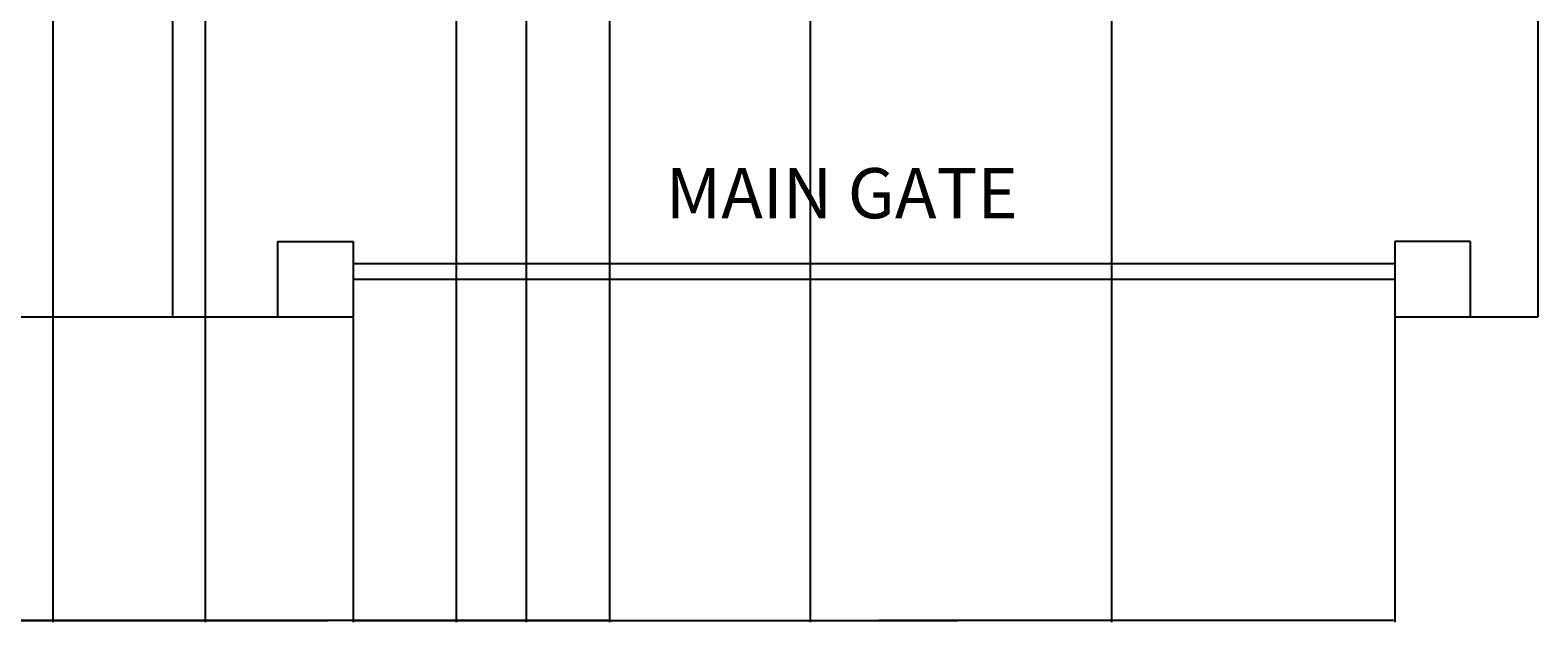
# Model space of a CAD drawing. Units: inches. Extents: x -36 to 401, y -686 to 73.
# Tile 3 of 15: x 184 to 365, y -686 to -615. Entities that reach past the tile are written whole.
import ezdxf

# ---------------------------------------------------------------- set-up
doc = ezdxf.new("R2010")
doc.units = ezdxf.units.IN
doc.header["$MEASUREMENT"] = 0
for name, color, linetype, lineweight in [('A-ANNO-DIMS', 2, 'Continuous', 18), ('A-ANNO-TEXT', 7, 'Continuous', 18), ('C-PROP', 7, 'Continuous', 25), ('C-SITE-GATE', 7, 'Continuous', 25)]:
    doc.layers.add(name, color=color, linetype=linetype, lineweight=lineweight)
doc.styles.get("Standard").update_dxf_attribs({"font": 'arial.ttf'})
doc.dimstyles.get("Standard").update_dxf_attribs({"dimtxt": 0.18, "dimasz": 0.18, "dimexe": 0.18, "dimexo": 0.0625, "dimgap": 0.09, "dimtad": 0, "dimtih": 1, "dimtoh": 1, "dimdec": 0, "dimzin": 0, "dimdsep": 46, "dimlunit": 3, "dimtxsty": 'Standard', "dimcen": 0.09, "dimadec": 0, "dimazin": 0, "dimtfac": 1, "dimtdec": 0, "dimtofl": 0, "dimtmove": 0, "dimatfit": 3, "dimfxl": 1, "dimtolj": 1, "dimtzin": 0, "dimarcsym": 0})

# ---------------------------------------------------------------- blocks, each defined once
blk = doc.blocks.new('*D3')
at = {"layer": 'A-ANNO-DIMS', "color": 0, "lineweight": -2, "transparency": 16777216}
for p, q in [((200.9, -421.21), (201.62, -421.21)), ((201.44, -421.39), (201.44, -532.06)), ((201.44, -649.03), (201.44, -538.36)), ((200.9, -649.21), (201.62, -649.21))]:
    blk.add_line(p, q, dxfattribs=at)
at = {"layer": 'A-ANNO-DIMS', "color": 0, "transparency": 16777216}
for points in [[(201.41, -421.39), (201.47, -421.39), (201.44, -421.21)], [(201.41, -649.03), (201.47, -649.03), (201.44, -649.21)]]:
    blk.add_solid(points, dxfattribs=at)
at = {"layer": 'Defpoints', "color": 0, "transparency": 16777216}
for p in [(200.84, -421.21), (200.84, -649.21), (201.44, -649.21)]:
    blk.add_point(p, dxfattribs=at)
at = {"layer": 'A-ANNO-DIMS', "color": 0, "transparency": 16777216, "insert": (201.44, -535.21), "char_height": 6, "attachment_point": 5}
blk.add_mtext("\\A1;19'", dxfattribs=at)
blk = doc.blocks.new('*D63')
at = {"layer": 'A-ANNO-DIMS', "color": 0, "lineweight": -2, "transparency": 16777216}
for p, q in [((223.02, -649.27), (223.02, -685.69)), ((347.59, -649.27), (347.59, -685.69)), ((223.2, -685.51), (284.7, -685.51)), ((347.41, -685.51), (285.9, -685.51))]:
    blk.add_line(p, q, dxfattribs=at)
at = {"layer": 'A-ANNO-DIMS', "color": 0, "transparency": 16777216}
for points in [[(223.2, -685.48), (223.2, -685.54), (223.02, -685.51)], [(347.41, -685.48), (347.41, -685.54), (347.59, -685.51)]]:
    blk.add_solid(points, dxfattribs=at)
at = {"layer": 'Defpoints', "color": 0, "transparency": 16777216}
for p in [(223.02, -649.21), (347.59, -649.21), (347.59, -685.51)]:
    blk.add_point(p, dxfattribs=at)
at = {"layer": 'A-ANNO-DIMS', "color": 0, "transparency": 16777216, "insert": (285.3, -685.51), "char_height": 0.18, "attachment_point": 5}
blk.add_mtext('\\A1;10\'-4 1/2"', dxfattribs=at)
blk = doc.blocks.new('*D64')
at = {"layer": 'A-ANNO-DIMS', "color": 0, "lineweight": -2, "transparency": 16777216}
for p, q in [((1.69, -649.27), (1.69, -685.69)), ((223.02, -649.27), (223.02, -685.69)), ((1.87, -685.51), (111.75, -685.51)), ((222.84, -685.51), (112.95, -685.51))]:
    blk.add_line(p, q, dxfattribs=at)
at = {"layer": 'A-ANNO-DIMS', "color": 0, "transparency": 16777216}
for points in [[(1.87, -685.48), (1.87, -685.54), (1.69, -685.51)], [(222.84, -685.48), (222.84, -685.54), (223.02, -685.51)]]:
    blk.add_solid(points, dxfattribs=at)
at = {"layer": 'Defpoints', "color": 0, "transparency": 16777216}
for p in [(1.69, -649.21), (223.02, -649.21), (223.02, -685.51)]:
    blk.add_point(p, dxfattribs=at)
at = {"layer": 'A-ANNO-DIMS', "color": 0, "transparency": 16777216, "insert": (112.35, -685.51), "char_height": 0.18, "attachment_point": 5}
blk.add_mtext('\\A1;18\'-5 1/2"', dxfattribs=at)
blk = doc.blocks.new('*D73')
at = {"layer": 'A-ANNO-DIMS', "color": 0, "lineweight": -2, "transparency": 16777216}
for p, q in [((177.19, -421.27), (177.19, -685.69)), ((253.69, -421.27), (253.69, -685.69)), ((177.37, -685.51), (214.9, -685.51)), ((253.51, -685.51), (215.98, -685.51))]:
    blk.add_line(p, q, dxfattribs=at)
at = {"layer": 'A-ANNO-DIMS', "color": 0, "transparency": 16777216}
for points in [[(177.37, -685.48), (177.37, -685.54), (177.19, -685.51)], [(253.51, -685.48), (253.51, -685.54), (253.69, -685.51)]]:
    blk.add_solid(points, dxfattribs=at)
at = {"layer": 'Defpoints', "color": 0, "transparency": 16777216}
for p in [(177.19, -421.21), (253.69, -421.21), (253.69, -685.51)]:
    blk.add_point(p, dxfattribs=at)
at = {"layer": 'A-ANNO-DIMS', "color": 0, "transparency": 16777216, "insert": (215.44, -685.51), "char_height": 0.18, "attachment_point": 5}
blk.add_mtext('\\A1;6\'-4 1/2"', dxfattribs=at)
blk = doc.blocks.new('*D74')
at = {"layer": 'A-ANNO-DIMS', "color": 0, "lineweight": -2, "transparency": 16777216}
for p, q in [((277.69, -412.27), (277.69, -685.69)), ((313.69, -421.27), (313.69, -685.69)), ((277.87, -685.51), (295.36, -685.51)), ((313.51, -685.51), (296.02, -685.51))]:
    blk.add_line(p, q, dxfattribs=at)
at = {"layer": 'A-ANNO-DIMS', "color": 0, "transparency": 16777216}
for points in [[(277.87, -685.48), (277.87, -685.54), (277.69, -685.51)], [(313.51, -685.48), (313.51, -685.54), (313.69, -685.51)]]:
    blk.add_solid(points, dxfattribs=at)
at = {"layer": 'Defpoints', "color": 0, "transparency": 16777216}
for p in [(277.69, -412.21), (313.69, -421.21), (313.69, -685.51)]:
    blk.add_point(p, dxfattribs=at)
at = {"layer": 'A-ANNO-DIMS', "color": 0, "transparency": 16777216, "insert": (295.69, -685.51), "char_height": 0.18, "attachment_point": 5}
blk.add_mtext('\\A1;3\'-0"', dxfattribs=at)
blk = doc.blocks.new('*D87')
at = {"layer": 'A-ANNO-DIMS', "color": 0, "lineweight": -2, "transparency": 16777216}
for p, q in [((243.7, -154.81), (243.7, -685.69)), ((187.11, -163.6), (187.11, -685.69)), ((187.29, -685.51), (214.86, -685.51)), ((243.52, -685.51), (215.95, -685.51))]:
    blk.add_line(p, q, dxfattribs=at)
at = {"layer": 'A-ANNO-DIMS', "color": 0, "transparency": 16777216}
for points in [[(187.29, -685.48), (187.29, -685.54), (187.11, -685.51)], [(243.52, -685.48), (243.52, -685.54), (243.7, -685.51)]]:
    blk.add_solid(points, dxfattribs=at)
at = {"layer": 'Defpoints', "color": 0, "transparency": 16777216}
for p in [(243.7, -154.75), (187.11, -163.53), (243.7, -685.51)]:
    blk.add_point(p, dxfattribs=at)
at = {"layer": 'A-ANNO-DIMS', "color": 0, "transparency": 16777216, "insert": (215.4, -685.51), "char_height": 0.18, "attachment_point": 5}
blk.add_mtext('\\A1;4\'-8 1/2"', dxfattribs=at)
blk = doc.blocks.new('*D91')
at = {"layer": 'A-ANNO-DIMS', "color": 0, "lineweight": -2, "transparency": 16777216}
for p, q in [((205.32, -404.21), (205.32, -685.69)), ((235.34, -404.21), (235.34, -685.69)), ((205.5, -685.51), (220, -685.51)), ((235.16, -685.51), (220.66, -685.51))]:
    blk.add_line(p, q, dxfattribs=at)
at = {"layer": 'A-ANNO-DIMS', "color": 0, "transparency": 16777216}
for points in [[(205.5, -685.48), (205.5, -685.54), (205.32, -685.51)], [(235.16, -685.48), (235.16, -685.54), (235.34, -685.51)]]:
    blk.add_solid(points, dxfattribs=at)
at = {"layer": 'Defpoints', "color": 0, "transparency": 16777216}
for p in [(205.32, -404.14), (235.34, -404.14), (235.34, -685.51)]:
    blk.add_point(p, dxfattribs=at)
at = {"layer": 'A-ANNO-DIMS', "color": 0, "transparency": 16777216, "insert": (220.33, -685.51), "char_height": 0.18, "attachment_point": 5}
blk.add_mtext('\\A1;2\'-6"', dxfattribs=at)

msp = doc.modelspace()

# ---------------------------------------------------------------- linework, layer by layer
at = {"layer": 'C-PROP'}
for p, q in [((364.69, 31.79), (364.69, -649.21)), ((1.69, -649.21), (223.02, -649.21)), ((347.59, -649.21), (364.69, -649.21))]:
    msp.add_line(p, q, dxfattribs=at)
at = {"layer": 'C-SITE-GATE'}
for p, q in [((214.02, -649.21), (214.02, -640.21)), ((214.02, -640.21), (223.02, -640.21)), ((223.02, -640.21), (223.02, -649.21)), ((356.59, -640.21), (347.59, -640.21)), ((347.59, -640.21), (347.59, -649.21)), ((356.59, -640.21), (356.59, -649.21)), ((347.59, -642.89), (223.02, -642.89)), ((223.02, -644.71), (347.59, -644.71))]:
    msp.add_line(p, q, dxfattribs=at)

# ---------------------------------------------------------------- texts
at = {"layer": 'A-ANNO-TEXT', "insert": (260.39, -631.43), "char_height": 6, "attachment_point": 1}
msp.add_mtext('MAIN GATE', dxfattribs=at)

# ---------------------------------------------------------------- dimensions: what is measured, and where the dimension line sits
at = {"layer": 'A-ANNO-DIMS'}
for base, p1, p2, picture, middle in [((243.7, -685.51), (187.11, -163.53), (243.7, -154.75), '*D87', (215.4, -685.51)), ((235.34, -685.51), (205.32, -404.14), (235.34, -404.14), '*D91', (220.33, -685.51)), ((313.69, -685.51), (277.69, -412.21), (313.69, -421.21), '*D74', (295.69, -685.51)), ((253.69, -685.51), (177.19, -421.21), (253.69, -421.21), '*D73', (215.44, -685.51)), ((223.02, -685.51), (1.69, -649.21), (223.02, -649.21), '*D64', (112.35, -685.51)), ((347.59, -685.51), (223.02, -649.21), (347.59, -649.21), '*D63', (285.3, -685.51))]:
    dim = msp.add_linear_dim(base=base, p1=p1, p2=p2, dimstyle='Standard', override={"dimdec": 1, "dimlfac": 1, "dimrnd": 0, "dimzin": 1, "dimdsep": 46, "dimlunit": 4, "dimfrac": 2}, dxfattribs=at)
    dim.commit()
    dim.dimension.update_dxf_attribs({"geometry": picture, "text_midpoint": middle})
dim = msp.add_linear_dim(base=(201.44, -649.21), p1=(200.84, -421.21), p2=(200.84, -649.21), angle=90, dimstyle='Standard', override={"dimtxt": 6, "dimclrd": 0, "dimclre": 0, "dimclrt": 0}, dxfattribs=at)
dim.commit()
dim.dimension.update_dxf_attribs({"geometry": '*D3', "text_midpoint": (201.44, -535.21)})

doc.saveas('drawing.dxf')
